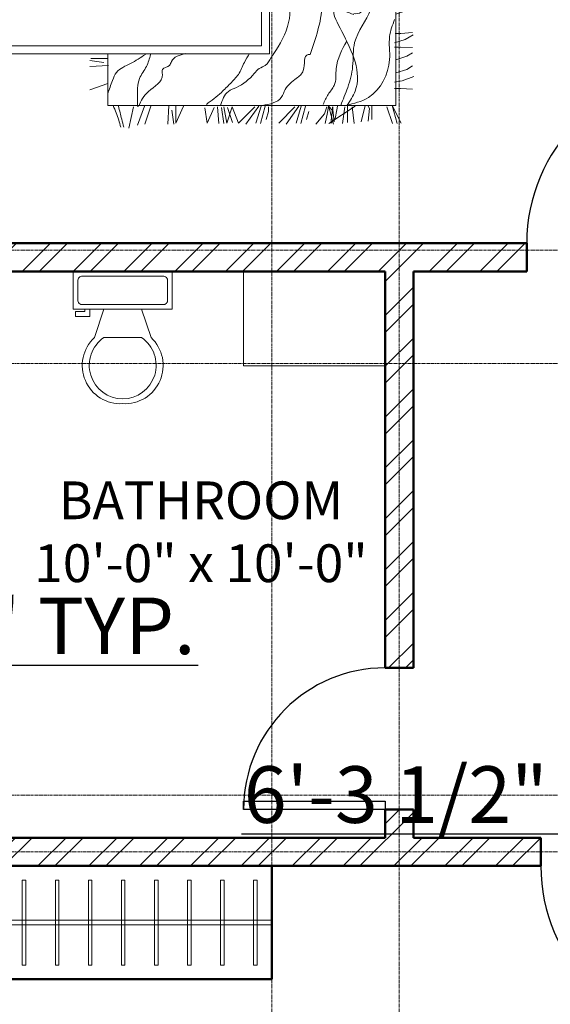
# Model space of a CAD drawing. Units: inches. Extents: x 261 to 2725, y 291 to 1454.
# Tile 21 of 35: x 1295 to 1407, y 644 to 853. Entities that reach past the tile are written whole.
import ezdxf

# ---------------------------------------------------------------- set-up
doc = ezdxf.new("R2010")
doc.units = ezdxf.units.IN
doc.linetypes.add('CENTER', pattern=[2, 1.25, -0.25, 0.25, -0.25])
for name, color, linetype, lineweight in [('A-ANNO-DIMS', 136, 'Continuous', 18), ('A-AREA-IDEN', 18, 'Continuous', 18), ('A-DOOR', 160, 'Continuous', 25), ('A-FLOR-FIXT', 145, 'Continuous', 18), ('A-FURN', 30, 'Continuous', 18), ('A-GRID', 251, 'CENTER', 13), ('A-WALL', 222, 'Continuous', 50), ('A-WALL-PATT', 243, 'Continuous', 13)]:
    doc.layers.add(name, color=color, linetype=linetype, lineweight=lineweight)
doc.styles.get("Standard").update_dxf_attribs({"font": 'arial.ttf'})
doc.dimstyles.new('ISO-25', dxfattribs={"dimtxt": 12, "dimasz": 6, "dimexe": 1.25, "dimexo": 0.625, "dimtad": 1, "dimdec": 0, "dimlunit": 3, "dimtxsty": 'Standard', "dimblk": 'ARCHTICK', "dimcen": 2.5, "dimadec": 0, "dimazin": 0, "dimtfac": 1, "dimtdec": 0, "dimtmove": 0, "dimatfit": 3, "dimfxl": 1, "dimfxlon": 1, "dimarcsym": 0})

# ---------------------------------------------------------------- blocks, each defined once
blk = doc.blocks.new('*U6')
for p, q in [((-36, 0), (-36, 6)), ((0, 0), (0, 6))]:
    blk.add_line(p, q)
blk.add_lwpolyline([(0, 0), (0, -36), (-1.75, -36), (-1.75, 0)], close=True)
blk.add_arc((0, 0), 36, 180, 270)
blk = doc.blocks.new('*U3')
for p, q in [((0, 0), (0, -6)), ((30, 0), (30, -6))]:
    blk.add_line(p, q)
blk.add_lwpolyline([(0, 0), (0, 30), (1.75, 30), (1.75, 0)], close=True)
blk.add_arc((0, 0), 30, 0, 90)
blk = doc.blocks.new('*U7')
for p, q in [((0, 0), (0, -6)), ((-36, 0), (-36, -6))]:
    blk.add_line(p, q)
blk.add_lwpolyline([(0, 0), (0, 36), (-1.75, 36), (-1.75, 0)], close=True)
blk.add_arc((0, 0), 36, 90, 180)
blk = doc.blocks.new('A$C2B723114')
for p, q in [((0, 2.9047), (2.8274, 2.9047)), ((0, 2.8487), (0, 2.9047)), ((2.8274, 2.9047), (2.8274, 2.8487)), ((2.8274, 2.8487), (0, 2.8487)), ((0.1012, 2.4649), (0.1012, 2.849)), ((0.1396, 2.5033), (0.1396, 2.849)), ((0.4243, 2.8697), (0.4243, 2.4855)), ((0.6794, 0.7051), (0.6794, 2.8509)), ((0.7187, 0.7435), (0.7187, 2.8509)), ((2.1776, 2.8509), (2.1776, 0.7454)), ((2.216, 2.8509), (2.216, 0.707)), ((2.4742, 2.8697), (2.4742, 2.4855)), ((2.6798, 2.5052), (2.6798, 2.8509)), ((2.7182, 2.4668), (2.7182, 2.8509)), ((0.6087, 2.6776), (0.295, 2.6776)), ((2.6586, 2.6776), (2.2821, 2.6776)), ((1.3789, 2.4999), (1.3598, 2.5761)), ((2.0593, 2.4999), (2.0402, 2.5761)), ((0.6766, 2.5033), (0.1396, 2.5033)), ((1.3858, 2.4723), (1.3789, 2.4999)), ((2.0662, 2.4723), (2.0593, 2.4999)), ((2.2188, 2.5052), (2.6798, 2.5052)), ((0.6794, 2.4649), (0.1012, 2.4649)), ((0.7191, 2.47), (2.1778, 2.4719)), ((2.2188, 2.4668), (2.7182, 2.4668)), ((2.1771, 2.3036), (0.718, 2.1685)), ((1.0365, 1.6233), (2.1246, 2.2989)), ((2.2287, 1.6076), (2.2523, 1.5035)), ((2.2726, 1.593), (2.3061, 1.5007)), ((2.3067, 1.5881), (2.3373, 1.5007)), ((2.4194, 1.5881), (2.4251, 1.4979)), ((2.4487, 1.5881), (2.4389, 1.5199)), ((0.5047, 1.5819), (0.5353, 1.4945)), ((0.6174, 1.5819), (0.6232, 1.4916)), ((0.6467, 1.5819), (0.6369, 1.5137)), ((0.6571, 1.4945), (0.6571, 1.5765)), ((2.4591, 1.5007), (2.4591, 1.5828)), ((0.4269, 0.0884), (0.4269, 1.4945)), ((0.4269, 1.4945), (0.6794, 1.4945)), ((2.4685, 1.4964), (2.216, 1.5022)), ((2.4685, 1.4964), (2.4685, 0.0903)), ((2.4685, 1.4044), (2.5491, 1.3861)), ((0.3172, 1.3923), (0.4213, 1.3687)), ((0.3318, 1.3485), (0.4241, 1.3149)), ((2.4596, 1.3659), (2.552, 1.3324)), ((0.3367, 1.3143), (0.4241, 1.2838)), ((2.4645, 1.3318), (2.552, 1.3012)), ((2.4645, 1.2928), (2.5548, 1.2871)), ((2.4645, 1.2635), (2.5328, 1.2733)), ((2.4699, 1.2531), (2.552, 1.2163)), ((2.552, 1.2531), (2.4699, 1.2531)), ((2.5435, 1.2276), (2.4699, 1.2163)), ((2.4699, 1.2163), (2.5463, 1.1823)), ((0.3367, 1.2016), (0.427, 1.1959)), ((0.3367, 1.1724), (0.405, 1.1821)), ((0.4241, 1.162), (0.3421, 1.162)), ((0.3421, 1.162), (0.4241, 1.1252)), ((2.5491, 1.1654), (2.467, 1.1597)), ((2.5463, 1.1455), (2.467, 1.1342)), ((2.5491, 1.1342), (2.4699, 1.1201)), ((2.4699, 1.1201), (2.5491, 1.0946)), ((2.5463, 1.1172), (2.4727, 1.0918)), ((2.5491, 1.0946), (2.4699, 1.0635)), ((2.4699, 1.0635), (2.5491, 0.9842)), ((0.4157, 1.0206), (0.3421, 1.0093)), ((2.4642, 1.0267), (2.552, 0.9644)), ((0.3421, 1.0093), (0.4185, 0.9754)), ((2.4699, 0.9785), (2.552, 0.9531)), ((0.4213, 0.9584), (0.3392, 0.9527)), ((0.4185, 0.9386), (0.3392, 0.9272)), ((0.4213, 0.9272), (0.3421, 0.9131)), ((2.4642, 0.9389), (2.4869, 0.9276)), ((2.467, 0.9559), (2.552, 0.9333)), ((2.4869, 0.9276), (2.5265, 0.9163)), ((2.5265, 0.9163), (2.5491, 0.9163)), ((0.3421, 0.9131), (0.4213, 0.8876)), ((0.4213, 0.8876), (0.3421, 0.8565)), ((0.4185, 0.9103), (0.3449, 0.8848)), ((2.4642, 0.8908), (2.5152, 0.8483)), ((0.3364, 0.8197), (0.4241, 0.7574)), ((0.3421, 0.8565), (0.4213, 0.7772)), ((2.467, 0.8455), (2.5208, 0.8342)), ((2.5152, 0.8483), (2.5491, 0.837)), ((2.5208, 0.8342), (2.552, 0.8285)), ((2.552, 0.8285), (2.5293, 0.8087)), ((0.3421, 0.7716), (0.4241, 0.7461)), ((2.5491, 0.7606), (2.467, 0.7719)), ((2.4699, 0.8172), (2.4925, 0.7974)), ((2.5491, 0.8087), (2.4699, 0.8172)), ((2.4925, 0.7974), (2.535, 0.7889)), ((2.535, 0.7889), (2.552, 0.7861)), ((0.3392, 0.7489), (0.4241, 0.7263)), ((2.1776, 0.7454), (0.7187, 0.7435)), ((2.4727, 0.7464), (2.467, 0.7408)), ((2.467, 0.7153), (2.5491, 0.7238)), ((2.552, 0.7464), (2.4727, 0.7464)), ((0.359, 0.7206), (0.3987, 0.7093)), ((0.3987, 0.7093), (0.4213, 0.7093)), ((2.216, 0.707), (0.6794, 0.7051)), ((0.9938, 0.6115), (1.7555, 0.7064)), ((2.5491, 0.6842), (2.4642, 0.6615)), ((2.552, 0.7096), (2.467, 0.6842)), ((0.3421, 0.6601), (0.4213, 0.5808)), ((2.5491, 0.6672), (2.4755, 0.6587)), ((2.4755, 0.6474), (2.5548, 0.6276)), ((0.3364, 0.6233), (0.4241, 0.561)), ((2.4642, 0.6191), (2.4784, 0.6134)), ((2.467, 0.5993), (2.4869, 0.5964)), ((2.4784, 0.6134), (2.5406, 0.6077)), ((2.4869, 0.5964), (2.552, 0.5964)), ((2.5406, 0.6077), (2.552, 0.6134)), ((0.3392, 0.5525), (0.4241, 0.5299)), ((0.3421, 0.5752), (0.4241, 0.5497)), ((2.467, 0.5313), (2.5491, 0.5596)), ((2.467, 0.5087), (2.5548, 0.5342)), ((2.5548, 0.5342), (2.4699, 0.4889)), ((0.359, 0.5242), (0.3987, 0.5129)), ((1.4523, 0.5021), (1.1305, 0.4537)), ((0.3364, 0.4785), (0.3874, 0.436)), ((0.3392, 0.4332), (0.393, 0.4219)), ((0.3874, 0.436), (0.4213, 0.4247)), ((1.1305, 0.4537), (0.9938, 0.448)), ((0.4213, 0.415), (0.3364, 0.3923)), ((0.4241, 0.2868), (0.3392, 0.415)), ((0.3421, 0.4049), (0.3647, 0.3851)), ((0.4213, 0.3964), (0.3421, 0.4049)), ((0.4213, 0.398), (0.3477, 0.3895)), ((0.3647, 0.3851), (0.4072, 0.3766)), ((0.393, 0.4219), (0.4241, 0.4162)), ((0.4241, 0.4162), (0.4015, 0.3964)), ((2.467, 0.4133), (2.552, 0.4019)), ((2.467, 0.2879), (2.552, 0.4076)), ((0.4213, 0.3377), (0.3392, 0.3491)), ((0.4072, 0.3766), (0.4241, 0.3738)), ((0.3392, 0.2925), (0.4213, 0.3009)), ((0.4241, 0.3236), (0.3449, 0.3236)), ((2.4642, 0.3049), (2.5491, 0.2851)), ((2.467, 0.319), (2.5548, 0.3134)), ((0.3477, 0.2571), (0.427, 0.2373)), ((2.4699, 0.2491), (2.501, 0.2491)), ((2.501, 0.2491), (2.5491, 0.2547)), ((0.3506, 0.2231), (0.4128, 0.2175)), ((0.359, 0.2061), (0.4241, 0.2061)), ((0.4128, 0.2175), (0.4241, 0.2231)), ((2.467, 0.2179), (2.5605, 0.1981)), ((2.467, 0.1981), (2.5491, 0.1613)), ((2.467, 0.184), (2.4982, 0.1755)), ((2.4982, 0.1755), (2.5463, 0.1359)), ((0.3392, 0.1042), (0.4213, 0.1325)), ((0.3392, 0.0815), (0.427, 0.107)), ((0.427, 0.107), (0.3421, 0.0617)), ((1.5674, 0.0962), (1.5844, 0.0453)), ((1.8568, 0.0962), (1.8738, 0.0453)), ((1.9342, 0.0962), (1.9512, 0.0453)), ((2.2236, 0.0962), (2.2406, 0.0453)), ((2.4642, 0.0991), (2.5378, 0.0877)), ((2.4699, 0.1302), (2.535, 0.1104)), ((2.535, 0.1104), (2.5491, 0.0991)), ((2.4685, 0.0903), (0.4269, 0.0884)), ((0.5106, 0.0657), (0.5077, 0.0063)), ((0.5106, 0.094), (0.5106, 0.0657)), ((0.5417, 0.094), (0.5474, 0.0572)), ((0.5474, 0.0572), (0.57, 0.0006)), ((0.587, 0.0884), (0.604, 0.0346)), ((0.6512, 0.0884), (0.6682, 0.0346)), ((0.713, 0.0657), (0.7101, 0.0063)), ((0.713, 0.094), (0.713, 0.0657)), ((0.7334, 0.0943), (0.7503, 0.0434)), ((0.7786, 0.0915), (0.7786, 0.0632)), ((0.7786, 0.0632), (0.7843, 0.0066)), ((0.8739, 0.0884), (0.8908, 0.0346)), ((0.956, 0.0943), (0.973, 0.0434)), ((1.0013, 0.0915), (1.0013, 0.0632)), ((1.0013, 0.0632), (1.007, 0.0066)), ((1.072, 0.0884), (1.089, 0.0346)), ((1.1338, 0.0657), (1.131, 0.0063)), ((1.1338, 0.094), (1.1338, 0.0657)), ((1.1542, 0.0943), (1.1712, 0.0434)), ((1.1995, 0.0915), (1.1995, 0.0632)), ((1.1995, 0.0632), (1.2052, 0.0066)), ((1.4088, 0.0657), (1.406, 0.0063)), ((1.4088, 0.094), (1.4088, 0.0657)), ((1.44, 0.094), (1.4456, 0.0572)), ((1.4456, 0.0572), (1.4683, 0.0006)), ((1.4853, 0.0884), (1.5023, 0.0346)), ((1.6127, 0.0934), (1.6127, 0.0651)), ((1.6127, 0.0651), (1.6184, 0.0085)), ((1.6297, 0.0849), (1.624, 0.0028)), ((1.6693, 0.0623), (1.6608, 0.0028)), ((1.6721, 0.0877), (1.6693, 0.0623)), ((1.7344, 0.0651), (1.7316, 0.0057)), ((1.7344, 0.0934), (1.7344, 0.0651)), ((1.7655, 0.0934), (1.7712, 0.0566)), ((1.7712, 0.0566), (1.7938, 0)), ((1.8108, 0.0877), (1.8278, 0.034)), ((1.9795, 0.0934), (1.9795, 0.0651)), ((1.9795, 0.0651), (1.9852, 0.0085)), ((1.9965, 0.0849), (1.9908, 0.0028)), ((2.0361, 0.0623), (2.0276, 0.0028)), ((2.039, 0.0877), (2.0361, 0.0623)), ((2.1012, 0.0651), (2.0984, 0.0057)), ((2.1012, 0.0934), (2.1012, 0.0651)), ((2.1324, 0.0934), (2.138, 0.0566)), ((2.138, 0.0566), (2.1607, 0)), ((2.1777, 0.0877), (2.1946, 0.034)), ((2.2689, 0.0934), (2.2689, 0.0651)), ((2.2689, 0.0651), (2.2746, 0.0085)), ((2.2859, 0.0849), (2.2802, 0.0028)), ((2.3255, 0.0623), (2.317, 0.0028)), ((2.3284, 0.0877), (2.3255, 0.0623)), ((2.3906, 0.0651), (2.3878, 0.0057)), ((2.3906, 0.0934), (2.3906, 0.0651)), ((2.4218, 0.0934), (2.4274, 0.0566)), ((2.4274, 0.0566), (2.4501, 0)), ((2.467, 0.0877), (2.484, 0.034)), ((2.5378, 0.0877), (2.5463, 0.0821)), ((0.604, 0.0346), (0.621, 0.0063)), ((0.6682, 0.0346), (0.6851, 0.0063)), ((0.7503, 0.0434), (0.773, 0.0037)), ((0.8908, 0.0346), (0.9078, 0.0063)), ((0.973, 0.0434), (0.9957, 0.0037)), ((1.089, 0.0346), (1.106, 0.0063)), ((1.1712, 0.0434), (1.1939, 0.0037)), ((1.5023, 0.0346), (1.5192, 0.0082)), ((1.5844, 0.0453), (1.607, 0.0057)), ((1.8278, 0.034), (1.8448, 0.0057)), ((1.8738, 0.0453), (1.8964, 0.0057)), ((1.9512, 0.0453), (1.9739, 0.0057)), ((2.1946, 0.034), (2.2116, 0.0057)), ((2.2406, 0.0453), (2.2632, 0.0057)), ((2.484, 0.034), (2.501, 0.0057))]:
    blk.add_line(p, q)
for centre, radius in [((0.4243, 2.6776), 0.0821), ((2.4742, 2.6776), 0.0821), ((0.4243, 2.6776), 0.0493), ((2.4742, 2.6776), 0.0493)]:
    blk.add_circle(centre, radius)
for centre, radius, start, end in [((0.8078, 2.821), 0.00214, 160.436, 281.8931), ((0.8088, 2.8207), 0.00315, 111.7883, 160.436), ((0.8162, 2.8021), 0.0232, 94.3025, 111.7883), ((0.8091, 2.8151), 0.00394, 21.9904, 101.8931), ((0.8409, 2.7949), 0.0302, 158.579, 188.1335), ((1.0356, 2.8227), 0.2268, 188.1335, 192.1095), ((0.7994, 2.8112), 0.0144, 338.579, 21.9904), ((0.8165, 2.7987), 0.0266, 59.3487, 94.3025), ((0.8554, 2.8643), 0.0497, 239.3487, 264.7408), ((0.9202, 3.5684), 0.7568, 264.7408, 268.0921), ((0.8679, 2.7254), 0.0915, 74.0648, 94.2159), ((0.8679, 2.7254), 0.0915, 53.9136, 74.0648), ((0.9409, 4.189), 1.3777, 268.0921, 270.5757), ((0.8679, 2.7254), 0.0915, 36.1766, 53.9136), ((0.86, 2.6097), 0.2158, 62.7604, 69.1397), ((0.9466, 3.6164), 0.8051, 270.5757, 274.8018), ((0.9263, 2.7386), 0.0708, 51.6114, 62.7604), ((0.7461, 2.511), 0.3611, 46.1885, 51.6114), ((1.0364, 2.548), 0.2671, 87.4614, 94.8018), ((1.042, 2.6745), 0.1405, 79.8101, 87.4614), ((1.1532, 3.2931), 0.488, 259.8101, 263.9133), ((1.204, 3.7695), 0.9671, 263.9133, 270), ((1.204, 3.4318), 0.6294, 270, 277.5469), ((1.2573, 3.0292), 0.2233, 277.5469, 285.744), ((1.3941, 2.5438), 0.281, 98.4372, 105.744), ((1.3747, 2.6748), 0.1486, 90, 98.4372), ((1.3713, 2.8186), 0.0315, 274.4002, 333.4195), ((1.3747, 2.74), 0.0833, 78.7276, 90), ((1.3886, 2.8099), 0.0121, 333.4195, 78.7276), ((1.4882, 2.821), 0.00214, 160.436, 281.8931), ((1.4892, 2.8207), 0.00315, 111.7883, 160.436), ((1.4966, 2.8021), 0.0232, 94.3025, 111.7883), ((1.4895, 2.8151), 0.00394, 21.9904, 101.8931), ((1.5213, 2.7949), 0.0302, 158.579, 188.1335), ((1.716, 2.8227), 0.2268, 188.1335, 192.1095), ((1.4798, 2.8112), 0.0144, 338.579, 21.9904), ((1.4969, 2.7987), 0.0266, 59.3487, 94.3025), ((1.5358, 2.8643), 0.0497, 239.3487, 264.7408), ((1.6006, 3.5684), 0.7568, 264.7408, 268.0921), ((1.5483, 2.7254), 0.0915, 74.0648, 94.2159), ((1.5483, 2.7254), 0.0915, 53.9136, 74.0648), ((1.6213, 4.189), 1.3777, 268.0921, 270.5757), ((1.5483, 2.7254), 0.0915, 36.1766, 53.9136), ((1.5404, 2.6097), 0.2158, 62.7604, 69.1397), ((1.627, 3.6164), 0.8051, 270.5757, 274.8018), ((1.6067, 2.7386), 0.0708, 51.6114, 62.7604), ((1.4265, 2.511), 0.3611, 46.1885, 51.6114), ((1.7168, 2.548), 0.2671, 87.4614, 94.8018), ((1.7224, 2.6745), 0.1405, 79.8101, 87.4614), ((1.8336, 3.2931), 0.488, 259.8101, 263.9133), ((1.8844, 3.7695), 0.9671, 263.9133, 270), ((1.8844, 3.4318), 0.6294, 270, 277.5469), ((1.9377, 3.0292), 0.2233, 277.5469, 285.744), ((2.0745, 2.5438), 0.281, 98.4372, 105.744), ((2.0551, 2.6748), 0.1486, 90, 98.4372), ((2.0517, 2.8186), 0.0315, 274.4002, 333.4195), ((2.0551, 2.74), 0.0833, 78.7276, 90), ((2.069, 2.8099), 0.0121, 333.4195, 78.7276), ((0.635, 2.7368), 0.1829, 7.6809, 12.1095), ((-0.0181, 2.6487), 0.8418, 3.3687, 7.6809), ((0.8679, 2.7254), 0.0915, 18.4397, 36.1766), ((0.8523, 2.6218), 0.2076, 39.0349, 46.1885), ((0.9783, 2.7239), 0.0455, 28.3168, 39.0349), ((0.8558, 2.6579), 0.1846, 23.0028, 28.3168), ((0.923, 2.7382), 0.4535, 0, 6.2324), ((1.3154, 2.7368), 0.1829, 7.6809, 12.1095), ((0.6623, 2.6487), 0.8418, 3.3687, 7.6809), ((1.5483, 2.7254), 0.0915, 18.4397, 36.1766), ((1.5327, 2.6218), 0.2076, 39.0349, 46.1885), ((1.6587, 2.7239), 0.0455, 28.3168, 39.0349), ((1.5362, 2.6579), 0.1846, 23.0028, 28.3168), ((1.6034, 2.7382), 0.4535, 0, 6.2324), ((0.1976, 2.6614), 0.6258, 358.3669, 3.3687), ((0.5722, 2.8434), 0.8132, 347.8016, 350.3156), ((1.1884, 2.7382), 0.1881, 350.3156, 0), ((0.878, 2.6614), 0.6258, 358.3669, 3.3687), ((1.2526, 2.8434), 0.8132, 347.8016, 350.3156), ((1.8688, 2.7382), 0.1881, 350.3156, 0), ((1.9648, 2.5659), 0.6074, 171.9949, 177.3351), ((1.6528, 2.6098), 0.2924, 167.8016, 171.9949), ((2.6452, 2.5659), 0.6074, 171.9949, 177.3351), ((2.3332, 2.6098), 0.2924, 167.8016, 171.9949), ((-11.7321, 3.2823), 12.5718, 356.49514, 356.94504), ((-0.4351, 2.6794), 1.2587, 356.945, 358.3669), ((-11.0517, 3.2823), 12.5718, 356.49514, 356.94504), ((0.2453, 2.6794), 1.2587, 356.945, 358.3669), ((1.4204, 2.5912), 0.0624, 177.3351, 194.0452), ((2.1008, 2.5912), 0.0624, 177.3351, 194.0452), ((0.5206, 2.5319), 0.2961, 350.0016, 356.4951), ((1.4917, 3.1364), 0.681, 244.6889, 246.5156), ((1.4917, 3.1364), 0.681, 246.5156, 248.3423), ((1.4917, 3.1364), 0.681, 248.3423, 250.572), ((1.201, 2.5319), 0.2961, 350.0016, 356.4951), ((2.1721, 3.1364), 0.681, 244.6889, 246.5156), ((2.1721, 3.1364), 0.681, 246.5156, 248.3423), ((2.1721, 3.1364), 0.681, 248.3423, 250.572), ((0.8298, 2.4774), 0.0178, 170.0016, 196.6978), ((0.8139, 2.4726), 0.00122, 196.6978, 277.1204), ((0.8041, 2.5514), 0.0807, 277.1204, 286.2212), ((0.8068, 2.5419), 0.0707, 286.2212, 297.2841), ((0.8584, 2.4419), 0.0418, 102.869, 117.2841), ((0.879, 2.3515), 0.1345, 93.574, 102.869), ((0.9376, 1.4146), 1.0732, 90.2865, 93.574), ((0.9586, -2.7845), 5.2724, 89.0296, 90.2865), ((0.9954, -0.6123), 3.0999, 87.3904, 89.0296), ((1.0854, 1.364), 1.1216, 85.3824, 87.3904), ((1.28, 3.7729), 1.2952, 265.3824, 267.2509), ((1.228, 2.691), 0.2121, 267.2509, 281.5586), ((1.4917, 3.1364), 0.681, 250.572, 252.8018), ((1.2975, 2.3514), 0.1345, 83.5659, 101.5586), ((1.3002, 2.3754), 0.1104, 72.6136, 83.5659), ((1.3965, 2.6828), 0.2118, 252.6136, 260.5159), ((1.4027, 2.7202), 0.2496, 260.5159, 265.9171), ((1.385, 2.4721), 0.000845, 265.9171, 14.0449), ((1.5102, 2.4774), 0.0178, 170.0016, 196.6978), ((1.4943, 2.4726), 0.00122, 196.6978, 277.1204), ((1.4845, 2.5514), 0.0807, 277.1204, 286.2212), ((1.4872, 2.5419), 0.0707, 286.2212, 297.2841), ((1.5388, 2.4419), 0.0418, 102.869, 117.2841), ((1.5594, 2.3515), 0.1345, 93.574, 102.869), ((1.618, 1.4146), 1.0732, 90.2865, 93.574), ((1.639, -2.7845), 5.2724, 89.0296, 90.2865), ((1.6758, -0.6123), 3.0999, 87.3904, 89.0296), ((1.7658, 1.364), 1.1216, 85.3824, 87.3904), ((1.9604, 3.7729), 1.2952, 265.3824, 267.2509), ((1.9084, 2.691), 0.2121, 267.2509, 281.5586), ((2.1721, 3.1364), 0.681, 250.572, 252.8018), ((1.9779, 2.3514), 0.1345, 83.5659, 101.5586), ((1.9806, 2.3754), 0.1104, 72.6136, 83.5659), ((2.0769, 2.6828), 0.2118, 252.6136, 260.5159), ((2.0831, 2.7202), 0.2496, 260.5159, 265.9171), ((2.0654, 2.4721), 0.000845, 265.9171, 14.0449)]:
    blk.add_arc(centre, radius, start, end)
blk.add_ellipse((0.4962, 1.9132), major_axis=(0.4887, -0.4605), ratio=0.503305, start_param=0.491272, end_param=1.591113)
for points, knots in [([(0.6768, 1.3104), (0.6615, 1.3339), (0.6315, 1.3797), (0.604, 1.4501), (0.5417, 1.4748), (0.5064, 1.4871), (0.4848, 1.4945)], [0, 0, 0, 0, 110.980521, 216.571322, 273.316778, 363.252298, 363.252298, 363.252298, 363.252298]), ([(0.427, 1.4678), (0.4036, 1.4582), (0.3693, 1.4441), (0.3335, 1.4344), (0.3221, 1.4313)], [0, 0, 0, 0, 98.452083, 144.639601, 144.639601, 144.639601, 144.639601]), ([(0.4241, 1.4423), (0.4031, 1.437), (0.3691, 1.4284), (0.3351, 1.4199), (0.3221, 1.4167)], [0, 0, 0, 0, 84.638756, 136.955563, 136.955563, 136.955563, 136.955563]), ([(2.5548, 1.4853), (2.5314, 1.4757), (2.5031, 1.4641), (2.4737, 1.4555), (2.4685, 1.454)], [0, 0, 0, 0, 98.452083, 119.481049, 119.481049, 119.481049, 119.481049]), ([(2.552, 1.4598), (2.5309, 1.4545), (2.5031, 1.4475), (2.4753, 1.4406), (2.4685, 1.4389)], [0, 0, 0, 0, 84.638756, 111.94623, 111.94623, 111.94623, 111.94623]), ([(2.2145, 1.4211), (2.233, 1.4246), (2.2636, 1.4303), (2.2761, 1.3837), (2.3429, 1.3967), (2.3949, 1.3342), (2.4474, 1.3031), (2.4698, 1.2898)], [0, 0, 0, 0, 61.886907, 102.717887, 145.699352, 284.082577, 386.765171, 386.765171, 386.765171, 386.765171]), ([(0.6768, 1.286), (0.6567, 1.2911), (0.6145, 1.3017), (0.5543, 1.3533), (0.4816, 1.349), (0.4362, 1.3493), (0.4233, 1.3493)], [0, 0, 0, 0, 80.250278, 168.388677, 295.908361, 346.663112, 346.663112, 346.663112, 346.663112]), ([(0.4233, 1.3445), (0.4367, 1.3385), (0.464, 1.3264), (0.5129, 1.2848), (0.5456, 1.2161), (0.6131, 1.2349), (0.6142, 1.1913), (0.6642, 1.1806), (0.674, 1.144), (0.6817, 1.1154)], [0, 0, 0, 0, 56.745495, 115.23739, 254.956954, 286.678662, 337.828324, 366.201072, 468.500395, 468.500395, 468.500395, 468.500395]), ([(2.2145, 1.319), (2.2295, 1.319), (2.2678, 1.3192), (2.3288, 1.2705), (2.4143, 1.279), (2.4535, 1.2403), (2.4662, 1.2278)], [0, 0, 0, 0, 57.155505, 146.33427, 287.936209, 355.396728, 355.396728, 355.396728, 355.396728]), ([(2.2182, 1.2059), (2.2419, 1.1958), (2.3116, 1.1659), (2.342, 1.0552), (2.4266, 1.0223), (2.4474, 0.9811), (2.462, 0.9684), (2.4698, 0.9616)], [0, 0, 0, 0, 97.73655, 287.59661, 389.176293, 423.403759, 463.679181, 463.679181, 463.679181, 463.679181]), ([(2.3573, 1.127), (2.3656, 1.1759), (2.3758, 1.2352), (2.3371, 1.1853), (2.3602, 1.1713), (2.3768, 1.1612)], [0, 0, 0, 0, 107.853607, 130.728419, 189.220329, 189.220329, 189.220329, 189.220329]), ([(2.2145, 1.1476), (2.2246, 1.1286), (2.2575, 1.0666), (2.3612, 1.0009), (2.431, 0.9336), (2.4662, 0.8996)], [0, 0, 0, 0, 83.02987, 271.460712, 463.033803, 463.033803, 463.033803, 463.033803]), ([(0.6817, 0.8034), (0.6673, 0.8119), (0.6341, 0.8315), (0.5785, 0.8518), (0.5349, 0.8973), (0.4828, 0.9461), (0.4518, 0.9879), (0.4331, 1.013)], [0, 0, 0, 0, 65.318952, 150.437229, 226.833166, 307.58338, 429.454095, 429.454095, 429.454095, 429.454095]), ([(0.4282, 0.9448), (0.4547, 0.9353), (0.496, 0.9206), (0.5223, 0.8436), (0.5628, 0.7946), (0.6113, 0.7575), (0.6214, 0.7173), (0.6539, 0.7022), (0.672, 0.6897), (0.6768, 0.6864)], [0, 0, 0, 0, 102.299436, 159.044876, 303.717955, 348.579152, 391.138254, 454.581655, 477.456496, 477.456496, 477.456496, 477.456496]), ([(2.2145, 0.823), (2.227, 0.8201), (2.261, 0.8121), (2.261, 0.7401), (2.3352, 0.7659), (2.379, 0.6836), (2.4336, 0.6521), (2.4662, 0.6334)], [0, 0, 0, 0, 46.747668, 127.438174, 179.649794, 280.561838, 429.605131, 429.605131, 429.605131, 429.605131]), ([(0.4282, 0.74), (0.4347, 0.7029), (0.444, 0.6496), (0.5194, 0.6274), (0.555, 0.5807), (0.5975, 0.5243), (0.6789, 0.5415), (0.677, 0.5095), (0.6768, 0.5061)], [0, 0, 0, 0, 130.791737, 187.537266, 286.231946, 353.673191, 460.023761, 472.712403, 472.712403, 472.712403, 472.712403]), ([(2.2218, 0.7246), (2.2595, 0.716), (2.3548, 0.6945), (2.4265, 0.6268), (2.4698, 0.586)], [0, 0, 0, 0, 148.665024, 375.555892, 375.555892, 375.555892, 375.555892]), ([(0.6768, 0.6864), (0.7275, 0.655), (0.8251, 0.5944), (0.9391, 0.606), (0.9938, 0.6115)], [0, 0, 0, 0, 225.995823, 434.686543, 434.686543, 434.686543, 434.686543]), ([(2.3719, 0.6737), (2.3738, 0.6431), (2.3772, 0.5878), (2.3146, 0.6382), (2.3401, 0.7015), (2.2971, 0.6649), (2.2923, 0.6965), (2.289, 0.7176)], [0, 0, 0, 0, 83.446591, 150.887818, 201.642461, 230.015204, 286.760644, 286.760644, 286.760644, 286.760644]), ([(2.2145, 0.5167), (2.1764, 0.5522), (2.1051, 0.6184), (1.9357, 0.5803), (1.9385, 0.6342), (1.9388, 0.6395)], [0, 0, 0, 0, 208.073343, 389.01094, 409.01094, 409.01094, 409.01094, 409.01094]), ([(0.6768, 0.5061), (0.7554, 0.4794), (0.8591, 0.4442), (0.9675, 0.4473), (0.9938, 0.448)], [0, 0, 0, 0, 319.374611, 421.61723, 421.61723, 421.61723, 421.61723]), ([(0.4331, 0.4427), (0.4498, 0.4356), (0.4827, 0.4216), (0.5314, 0.3759), (0.632, 0.3884), (0.6996, 0.3513), (0.7423, 0.3278)], [0, 0, 0, 0, 70.931849, 139.556414, 248.154027, 434.709995, 434.709995, 434.709995, 434.709995]), ([(2.4625, 0.1088), (2.4095, 0.1438), (2.2904, 0.2226), (2.0623, 0.1771), (1.9006, 0.2246), (1.7699, 0.2337), (1.6941, 0.2766), (1.5528, 0.2786), (1.4005, 0.2587), (1.2324, 0.3267), (1.059, 0.2939), (0.9218, 0.426), (0.7359, 0.3204), (0.5586, 0.2391), (0.4502, 0.3116), (0.427, 0.3272)], [0, 0, 0, 0, 239.874704, 538.942419, 850.40885, 893.390315, 1047.998294, 1176.505142, 1437.500972, 1637.333004, 1864.324391, 2089.058767, 2248.736533, 2637.953392, 2744.252142, 2744.252142, 2744.252142, 2744.252142]), ([(1.9771, 0.0962), (1.9286, 0.1117), (1.7864, 0.157), (1.5223, 0.1992), (1.2611, 0.141), (1.0527, 0.2023), (0.8859, 0.1885), (0.76, 0.3042), (0.6211, 0.292), (0.5187, 0.3203), (0.4572, 0.3456), (0.4282, 0.3575)], [0, 0, 0, 0, 198.710624, 582.73994, 1031.873213, 1206.082894, 1423.278209, 1655.952104, 1808.744089, 1945.69963, 2068.229211, 2068.229211, 2068.229211, 2068.229211]), ([(0.8718, 0.2941), (0.8821, 0.3221), (0.9041, 0.3814), (0.9523, 0.2773), (0.8733, 0.2454), (0.8757, 0.2798), (0.8766, 0.2941)], [0, 0, 0, 0, 82.720021, 175.094899, 237.579423, 282.440623, 282.440623, 282.440623, 282.440623]), ([(0.8474, 0.0943), (0.82, 0.1047), (0.757, 0.1287), (0.6201, 0.1029), (0.4623, 0.1837), (0.4372, 0.2936), (0.4282, 0.3331)], [0, 0, 0, 0, 112.422038, 258.341957, 533.791494, 688.286079, 688.286079, 688.286079, 688.286079]), ([(1.2715, 0.221), (1.3344, 0.2172), (1.4529, 0.21), (1.2971, 0.2665), (1.2756, 0.2284), (1.2715, 0.221)], [0, 0, 0, 0, 150.888188, 283.977876, 315.699589, 315.699589, 315.699589, 315.699589])]:
    blk.add_open_spline(points, degree=3, knots=knots)
blk = doc.blocks.new('*U27')
for p, q in [((9.5, -6), (9.5, -2)), ((-8, -8.5), (-8, -8)), ((-7, -8), (-7, -9.5)), ((-4, -8), (-6, -14)), ((4, -8), (6, -14)), ((-10, -8.5), (-8, -8.5)), ((-10, -9.5), (-10, -8.5)), ((-7, -9.5), (-10, -9.5)), ((4, -14), (-4, -14))]:
    blk.add_line(p, q)
blk.add_lwpolyline([(10.5, -8), (10.5, 0), (-10.5, 0), (-10.5, -8)], close=True)
for points in [[(-9.5, -2), (-9.5, -6)], [(8.5, -1), (-8.5, -1)], [(-8.5, -7), (8.5, -7)]]:
    blk.add_lwpolyline(points)
for centre, radius, start, end in [((-8.625, -1.875), 0.8839, 81.8699, 188.1301), ((8.625, -1.875), 0.8839, 351.8699, 98.1301), ((-8.625, -6.125), 0.8839, 171.869898, 278.1301), ((8.625, -6.125), 0.8839, 261.8699, 8.1301), ((-0.4772, -19.9188), 8.0953, 133.01722, 273.38), ((0.0374, -19.8731), 7.127, 124.50543, 269.7), ((-0.0373, -19.8731), 7.127, 270.3, 55.4946), ((0.4773, -19.9188), 8.0953, 266.62, 46.9828)]:
    blk.add_arc(centre, radius, start, end)
blk = doc.blocks.new('_ArchTick')
at = {"color": 0, "linetype": 'ByBlock', "const_width": 0.15}
blk.add_lwpolyline([(-0.5, -0.5), (0.5, 0.5)], dxfattribs=at)
blk = doc.blocks.new('*D56')
at = {"layer": 'A-ANNO-DIMS', "color": 0, "lineweight": -2, "ltscale": 0.07, "transparency": 16777216}
for p, q in [((1450.08, 679.22), (1450.08, 681.47)), ((1525.71, 679.22), (1525.71, 681.47)), ((1450.08, 680.22), (1341.66, 680.22)), ((1525.71, 680.22), (1450.08, 680.22))]:
    blk.add_line(p, q, dxfattribs=at)
at = {"layer": 'Defpoints', "color": 0, "ltscale": 0.07, "transparency": 16777216}
for p in [(1450.08, 680.22), (1450.08, 664.47), (1525.71, 664.47)]:
    blk.add_point(p, dxfattribs=at)
at = {"layer": 'A-ANNO-DIMS', "color": 0, "lineweight": -2, "ltscale": 0.07, "transparency": 16777216, "xscale": 6, "yscale": 6, "zscale": 6, "rotation": 180}
blk.add_blockref('_ArchTick', (1450.08, 680.22), dxfattribs=at)
at = {"layer": 'A-ANNO-DIMS', "color": 0, "lineweight": -2, "ltscale": 0.07, "transparency": 16777216, "xscale": 6, "yscale": 6, "zscale": 6}
blk.add_blockref('_ArchTick', (1525.71, 680.22), dxfattribs=at)
at = {"layer": 'A-ANNO-DIMS', "color": 0, "ltscale": 0.07, "transparency": 16777216, "insert": (1392.87, 687.05), "char_height": 12, "attachment_point": 5}
blk.add_mtext('6\'-3 1/2" TYP.', dxfattribs=at)
blk = doc.blocks.new('*D60')
at = {"layer": 'A-ANNO-DIMS', "color": 0, "lineweight": -2, "ltscale": 0.07, "transparency": 16777216}
for p, q in [((1243.08, 717.07), (1243.08, 714.82)), ((1243.08, 716.07), (1252.08, 716.07)), ((1252.08, 717.07), (1252.08, 714.82)), ((1252.08, 716.07), (1332.48, 716.07))]:
    blk.add_line(p, q, dxfattribs=at)
at = {"layer": 'Defpoints', "color": 0, "ltscale": 0.07, "transparency": 16777216}
for p in [(1243.08, 721.47), (1252.08, 721.47), (1252.08, 716.07)]:
    blk.add_point(p, dxfattribs=at)
at = {"layer": 'A-ANNO-DIMS', "color": 0, "lineweight": -2, "ltscale": 0.07, "transparency": 16777216, "xscale": 6, "yscale": 6, "zscale": 6, "rotation": 180}
blk.add_blockref('_ArchTick', (1243.08, 716.07), dxfattribs=at)
at = {"layer": 'A-ANNO-DIMS', "color": 0, "lineweight": -2, "ltscale": 0.07, "transparency": 16777216, "xscale": 6, "yscale": 6, "zscale": 6}
blk.add_blockref('_ArchTick', (1252.08, 716.07), dxfattribs=at)
at = {"layer": 'A-ANNO-DIMS', "color": 0, "ltscale": 0.07, "transparency": 16777216, "insert": (1295.28, 722.82), "char_height": 12, "attachment_point": 5}
blk.add_mtext('0\'-9" TYP.', dxfattribs=at)
blk = doc.blocks.new('*D82')
at = {"layer": 'A-ANNO-DIMS', "color": 0, "lineweight": -2, "ltscale": 0.07, "transparency": 16777216}
for p, q in [((2600.96, 679.47), (2603.21, 679.47)), ((2601.96, 517.47), (2601.96, 679.47)), ((2600.96, 517.47), (2603.21, 517.47))]:
    blk.add_line(p, q, dxfattribs=at)
at = {"layer": 'Defpoints', "color": 0, "ltscale": 0.07, "transparency": 16777216}
for p in [(946.45, 679.47), (2601.96, 679.47), (946.45, 517.47)]:
    blk.add_point(p, dxfattribs=at)
at = {"layer": 'A-ANNO-DIMS', "color": 0, "lineweight": -2, "ltscale": 0.07, "transparency": 16777216, "xscale": 6, "yscale": 6, "zscale": 6}
for p, rotation in [((2601.96, 679.47), 90), ((2601.96, 517.47), 270)]:
    blk.add_blockref('_ArchTick', p, dxfattribs=dict(at, rotation=rotation))
at = {"layer": 'A-ANNO-DIMS', "color": 0, "ltscale": 0.07, "transparency": 16777216, "insert": (2595.2, 598.47), "char_height": 12, "attachment_point": 5, "rotation": 90}
blk.add_mtext('13\'-6"', dxfattribs=at)
blk = doc.blocks.new('*D83')
at = {"layer": 'A-ANNO-DIMS', "color": 0, "lineweight": -2, "ltscale": 0.07, "transparency": 16777216}
for p, q in [((2600.96, 799.47), (2603.21, 799.47)), ((2601.96, 679.47), (2601.96, 799.47)), ((2600.96, 679.47), (2603.21, 679.47))]:
    blk.add_line(p, q, dxfattribs=at)
at = {"layer": 'Defpoints', "color": 0, "ltscale": 0.07, "transparency": 16777216}
for p in [(946.45, 799.47), (2601.96, 799.47), (946.45, 679.47)]:
    blk.add_point(p, dxfattribs=at)
at = {"layer": 'A-ANNO-DIMS', "color": 0, "lineweight": -2, "ltscale": 0.07, "transparency": 16777216, "xscale": 6, "yscale": 6, "zscale": 6}
for p, rotation in [((2601.96, 799.47), 90), ((2601.96, 679.47), 270)]:
    blk.add_blockref('_ArchTick', p, dxfattribs=dict(at, rotation=rotation))
at = {"layer": 'A-ANNO-DIMS', "color": 0, "ltscale": 0.07, "transparency": 16777216, "insert": (2595.21, 739.47), "char_height": 12, "attachment_point": 5, "rotation": 90}
blk.add_mtext('10\'-0"', dxfattribs=at)
blk = doc.blocks.new('*D84')
at = {"layer": 'A-ANNO-DIMS', "color": 0, "lineweight": -2, "ltscale": 0.07, "transparency": 16777216}
for p, q in [((2600.96, 1024.47), (2603.21, 1024.47)), ((2601.96, 799.47), (2601.96, 1024.47)), ((2600.96, 799.47), (2603.21, 799.47))]:
    blk.add_line(p, q, dxfattribs=at)
at = {"layer": 'Defpoints', "color": 0, "ltscale": 0.07, "transparency": 16777216}
for p in [(946.45, 1024.47), (2601.96, 1024.47), (946.45, 799.47)]:
    blk.add_point(p, dxfattribs=at)
at = {"layer": 'A-ANNO-DIMS', "color": 0, "lineweight": -2, "ltscale": 0.07, "transparency": 16777216, "xscale": 6, "yscale": 6, "zscale": 6}
for p, rotation in [((2601.96, 1024.47), 90), ((2601.96, 799.47), 270)]:
    blk.add_blockref('_ArchTick', p, dxfattribs=dict(at, rotation=rotation))
at = {"layer": 'A-ANNO-DIMS', "color": 0, "ltscale": 0.07, "transparency": 16777216, "insert": (2595.21, 911.97), "char_height": 12, "attachment_point": 5, "rotation": 90}
blk.add_mtext('18\'-9"', dxfattribs=at)
blk = doc.blocks.new('*D121')
at = {"layer": 'A-ANNO-DIMS', "color": 0, "lineweight": -2, "ltscale": 0.07, "transparency": 16777216}
for p, q in [((1405.08, 305.22), (1405.08, 302.97)), ((1441.08, 305.22), (1441.08, 302.97)), ((1405.08, 304.22), (1441.08, 304.22))]:
    blk.add_line(p, q, dxfattribs=at)
at = {"layer": 'Defpoints', "color": 0, "ltscale": 0.07, "transparency": 16777216}
for p in [(1405.08, 673.47), (1441.08, 673.47), (1441.08, 304.22)]:
    blk.add_point(p, dxfattribs=at)
at = {"layer": 'A-ANNO-DIMS', "color": 0, "lineweight": -2, "ltscale": 0.07, "transparency": 16777216, "xscale": 6, "yscale": 6, "zscale": 6, "rotation": 180}
blk.add_blockref('_ArchTick', (1405.08, 304.22), dxfattribs=at)
at = {"layer": 'A-ANNO-DIMS', "color": 0, "lineweight": -2, "ltscale": 0.07, "transparency": 16777216, "xscale": 6, "yscale": 6, "zscale": 6}
blk.add_blockref('_ArchTick', (1441.08, 304.22), dxfattribs=at)
at = {"layer": 'A-ANNO-DIMS', "color": 0, "ltscale": 0.07, "transparency": 16777216, "insert": (1423.08, 310.97), "char_height": 12, "attachment_point": 5}
blk.add_mtext('3\'-0"', dxfattribs=at)
blk = doc.blocks.new('*D123')
at = {"layer": 'A-ANNO-DIMS', "color": 0, "lineweight": -2, "ltscale": 0.07, "transparency": 16777216}
for p, q in [((287.06, 1054.85), (284.81, 1054.85)), ((286.06, 439.47), (286.06, 1054.85)), ((287.06, 439.47), (284.81, 439.47))]:
    blk.add_line(p, q, dxfattribs=at)
at = {"layer": 'Defpoints', "color": 0, "ltscale": 0.07, "transparency": 16777216}
for p in [(286.06, 1054.85), (2007.71, 1054.85), (2007.71, 439.47)]:
    blk.add_point(p, dxfattribs=at)
at = {"layer": 'A-ANNO-DIMS', "color": 0, "lineweight": -2, "ltscale": 0.07, "transparency": 16777216, "xscale": 6, "yscale": 6, "zscale": 6}
for p, rotation in [((286.06, 1054.85), 90), ((286.06, 439.47), 270)]:
    blk.add_blockref('_ArchTick', p, dxfattribs=dict(at, rotation=rotation))
at = {"layer": 'A-ANNO-DIMS', "color": 0, "ltscale": 0.07, "transparency": 16777216, "insert": (279.22, 747.16), "char_height": 12, "attachment_point": 5, "rotation": 90}
blk.add_mtext('51\'-3 1/2"', dxfattribs=at)

msp = doc.modelspace()

# ---------------------------------------------------------------- hatches: boundary and pattern name
at = {"layer": 'A-WALL-PATT'}
h = msp.add_hatch(dxfattribs=at)
h.set_pattern_fill('ANSI32', color=256, scale=0.8)
h.paths.add_polyline_path([(478.45, 685.47), (580.45, 685.47), (580.45, 691.47), (577.45, 691.47), (577.45, 694.47), (571.45, 694.47), (571.45, 691.47), (478.45, 691.47), (478.45, 721.47), (469.45, 721.47), (469.45, 508.47), (538.45, 508.47), (538.45, 517.47), (478.45, 517.47)])
h.paths.add_polyline_path([(694.45, 517.47), (676.45, 517.47), (676.45, 646.47), (670.45, 646.47), (670.45, 517.47), (610.45, 517.47), (610.45, 508.47), (694.45, 508.47)])
h.paths.add_polyline_path([(676.45, 784.47), (478.45, 784.47), (478.45, 844.47), (469.45, 844.47), (469.45, 745.47), (478.45, 745.47), (478.45, 775.47), (571.45, 775.47), (571.45, 724.47), (577.45, 724.47), (577.45, 775.47), (670.45, 775.47), (670.45, 691.47), (610.45, 691.47), (610.45, 685.47), (670.45, 685.47), (670.45, 682.47), (676.45, 682.47)])
h.paths.add_polyline_path([(955.45, 880.47), (946.45, 880.47), (946.45, 808.47), (778.45, 808.47), (778.45, 799.47), (946.45, 799.47), (946.45, 517.47), (898.45, 517.47), (898.45, 508.47), (955.45, 508.47)])
h.paths.add_polyline_path([(778.45, 598.47), (772.45, 598.47), (772.45, 517.47), (754.45, 517.47), (754.45, 508.47), (826.45, 508.47), (826.45, 517.47), (778.45, 517.47)])
h.paths.add_polyline_path([(955.45, 1090.47), (946.45, 1090.47), (946.45, 1030.47), (817.45, 1030.47), (817.45, 1024.47), (946.45, 1024.47), (946.45, 952.47), (955.45, 952.47)])
h.paths.add_polyline_path([(955.45, 1231.47), (730.45, 1231.47), (730.45, 1222.47), (772.45, 1222.47), (772.45, 1096.47), (766.45, 1096.47), (766.45, 1090.47), (772.45, 1090.47), (772.45, 1006.47), (712.45, 1006.47), (712.45, 1000.47), (778.45, 1000.47), (778.45, 1024.47), (781.45, 1024.47), (781.45, 1030.47), (778.45, 1030.47), (778.45, 1222.47), (946.45, 1222.47), (946.45, 1162.47), (955.45, 1162.47)])
h.paths.add_polyline_path([(694.45, 1231.47), (619.45, 1231.47), (619.45, 1222.47), (646.45, 1222.47), (646.45, 1039.47), (652.45, 1039.47), (652.45, 1090.47), (736.45, 1090.47), (736.45, 1096.47), (652.45, 1096.47), (652.45, 1222.47), (694.45, 1222.47)])
h.paths.add_polyline_path([(571.45, 1231.47), (469.45, 1231.47), (469.45, 1099.47), (478.45, 1099.47), (478.45, 1144.47), (544.45, 1144.47), (544.45, 1153.47), (538.45, 1153.47), (538.45, 1150.47), (478.45, 1150.47), (478.45, 1222.47), (538.45, 1222.47), (538.45, 1183.47), (544.45, 1183.47), (544.45, 1222.47), (571.45, 1222.47)])
h.paths.add_polyline_path([(538.45, 1006.47), (478.45, 1006.47), (478.45, 1051.47), (469.45, 1051.47), (469.45, 940.47), (478.45, 940.47), (478.45, 1000.47), (538.45, 1000.47)])
h.paths.add_polyline_path([(652.45, 1006.47), (652.45, 1009.47), (646.45, 1009.47), (646.45, 1006.47), (586.45, 1006.47), (586.45, 1000.47), (652.45, 1000.47)])
h.paths.add_polyline_path([(1288.08, 973.47), (1243.08, 973.47), (1243.08, 920.97), (1252.08, 920.97), (1252.08, 964.47), (1288.08, 964.47)], flags=17)
h.paths.add_polyline_path([(1402.08, 805.47), (1252.08, 805.47), (1252.08, 848.97), (1243.08, 848.97), (1243.08, 757.47), (1252.08, 757.47), (1252.08, 799.47), (1294.08, 799.47), (1372.08, 799.47), (1372.08, 779.47), (1372.08, 715.47), (1378.08, 715.47), (1378.08, 799.47), (1402.08, 799.47)])
h.paths.add_polyline_path([(1252.08, 721.47), (1243.08, 721.47), (1243.08, 439.47), (1729.08, 439.47), (1729.08, 709.47), (1720.08, 709.47), (1720.08, 679.47), (1582.08, 679.47), (1582.08, 670.47), (1588.08, 670.47), (1588.08, 673.47), (1720.08, 673.47), (1720.08, 559.47), (1690.08, 559.47), (1690.08, 550.47), (1720.08, 550.47), (1720.08, 448.47), (1252.08, 448.47), (1252.08, 496.47), (1312.08, 496.47), (1312.08, 505.47), (1252.08, 505.47), (1252.08, 673.47), (1405.08, 673.47), (1405.08, 679.47), (1378.08, 679.47), (1378.08, 685.47), (1372.08, 685.47), (1372.08, 679.47), (1252.08, 679.47)])
h.paths.add_polyline_path([(1450.08, 550.47), (1480.08, 550.47), (1480.08, 559.47), (1450.08, 559.47), (1450.08, 679.47), (1441.08, 679.47), (1441.08, 673.47), (1444.08, 673.47), (1444.08, 505.47), (1384.08, 505.47), (1384.08, 496.47), (1450.08, 496.47)], flags=17)
h.paths.add_polyline_path([(1618.08, 559.47), (1588.08, 559.47), (1588.08, 634.47), (1582.08, 634.47), (1582.08, 559.47), (1552.08, 559.47), (1552.08, 550.47), (1618.08, 550.47)], flags=17)
h.paths.add_polyline_path([(1564.08, 964.47), (1630.08, 964.47), (1630.08, 973.47), (1477.08, 973.47), (1477.08, 964.47), (1558.08, 964.47), (1558.08, 926.22), (1558.08, 887.97), (1486.08, 887.97), (1486.08, 881.97), (1558.08, 881.97), (1558.08, 805.47), (1450.08, 805.47), (1450.08, 845.97), (1444.08, 845.97), (1444.08, 805.47), (1438.08, 805.47), (1438.08, 799.47), (1564.08, 799.47)], flags=17)
h.paths.add_polyline_path([(1453.08, 973.47), (1408.08, 973.47), (1408.08, 964.47), (1444.08, 964.47), (1444.08, 881.97), (1450.08, 881.97), (1456.08, 881.97), (1456.08, 887.97), (1450.08, 887.97), (1450.08, 964.47), (1453.08, 964.47)], flags=17)
h.paths.add_polyline_path([(1729.08, 1231.47), (1243.08, 1231.47), (1243.08, 1167.47), (1252.08, 1167.47), (1252.08, 1222.47), (1441.08, 1222.47), (1441.08, 1045.47), (1648.08, 1045.47), (1648.08, 1051.47), (1450.08, 1051.47), (1450.08, 1074.47), (1450.08, 1222.47), (1472.08, 1222.47), (1720.08, 1222.47), (1720.08, 1051.47), (1708.08, 1051.47), (1708.08, 1045.47), (1720.08, 1045.47), (1720.08, 973.47), (1702.08, 973.47), (1702.08, 964.47), (1720.08, 964.47), (1720.08, 769.47), (1729.08, 769.47)])
h.paths.add_polyline_path([(2493.71, 1054.85), (2007.71, 1054.85), (2007.71, 439.47), (2214.67, 439.47), (2214.67, 496.47), (2493.71, 496.47)])
h.paths.add_polyline_path([(2016.71, 1045.85), (2304.71, 1045.85), (2304.71, 841.47), (2310.71, 841.47), (2310.71, 1045.85), (2484.71, 1045.85), (2484.71, 805.47), (2310.71, 805.47), (2310.71, 811.47), (2304.71, 811.47), (2304.71, 799.47), (2484.71, 799.47), (2484.71, 679.47), (2304.71, 679.47), (2304.71, 673.47), (2484.71, 673.47), (2484.71, 505.47), (2208.67, 505.47), (2208.67, 448.47), (2016.71, 448.47), (2016.71, 799.47), (2304.71, 799.47), (2304.71, 805.47), (2016.71, 805.47)], flags=16)

# ---------------------------------------------------------------- linework, layer by layer
at = {"layer": 'A-FLOR-FIXT'}
msp.add_lwpolyline([(1342.08, 779.47), (1372.08, 779.47), (1372.08, 799.47), (1342.08, 799.47)], close=True, dxfattribs=at)
at = {"layer": 'A-FURN'}
for p, q in [((1348.08, 661.97), (1252.08, 661.97)), ((1348.08, 660.97), (1252.08, 660.97))]:
    msp.add_line(p, q, dxfattribs=at)
for points in [[(1295.2, 670.47), (1295.2, 652.47), (1295.95, 652.47), (1295.95, 670.47)], [(1302.2, 670.47), (1302.2, 652.47), (1302.95, 652.47), (1302.95, 670.47)], [(1309.2, 670.47), (1309.2, 652.47), (1309.95, 652.47), (1309.95, 670.47)], [(1316.2, 670.47), (1316.2, 652.47), (1316.95, 652.47), (1316.95, 670.47)], [(1323.2, 670.47), (1323.2, 652.47), (1323.95, 652.47), (1323.95, 670.47)], [(1330.2, 670.47), (1330.2, 652.47), (1330.95, 652.47), (1330.95, 670.47)], [(1337.2, 670.47), (1337.2, 652.47), (1337.95, 652.47), (1337.95, 670.47)], [(1344.2, 670.47), (1344.2, 652.47), (1344.95, 652.47), (1344.95, 670.47)]]:
    msp.add_lwpolyline(points, close=True, dxfattribs=at)
at = {"layer": 'A-GRID', "ltscale": 0.5}
for p, q in [((1348.08, 1330.18), (1348.08, 416.18)), ((1375.08, 1330.18), (1375.08, 416.18)), ((1167.93, 803.97), (1791.93, 803.97)), ((1167.93, 779.97), (1791.93, 779.97)), ((1167.93, 688.47), (1791.93, 688.47)), ((1167.93, 676.47), (1791.93, 676.47))]:
    msp.add_line(p, q, dxfattribs=at)
at = {"layer": 'A-WALL'}
for p, q in [((1252.08, 805.47), (1402.08, 805.47)), ((1402.08, 805.47), (1402.08, 799.47)), ((1252.08, 799.47), (1372.08, 799.47)), ((1372.08, 715.47), (1372.08, 799.47)), ((1378.08, 715.47), (1378.08, 799.47)), ((1378.08, 799.47), (1402.08, 799.47)), ((1378.08, 715.47), (1372.08, 715.47)), ((1372.08, 679.47), (1372.08, 685.47)), ((1378.08, 685.47), (1372.08, 685.47)), ((1378.08, 679.47), (1378.08, 685.47)), ((1252.08, 679.47), (1372.08, 679.47)), ((1378.08, 679.47), (1405.08, 679.47)), ((1405.08, 673.47), (1405.08, 679.47)), ((1252.08, 673.47), (1405.08, 673.47)), ((1348.08, 649.47), (1348.08, 673.47)), ((1252.08, 649.47), (1348.08, 649.47))]:
    msp.add_line(p, q, dxfattribs=at)

# ---------------------------------------------------------------- block references
at = {"layer": 'A-DOOR'}
for name, p in [('*U7', (1438.08, 805.47)), ('*U6', (1441.08, 673.47))]:
    msp.add_blockref(name, p, dxfattribs=at)
at = {"layer": 'A-DOOR', "rotation": 89.99999999999999}
msp.add_blockref('*U3', (1372.08, 685.47), dxfattribs=at)
at = {"layer": 'A-FLOR-FIXT'}
msp.add_blockref('*U27', (1316.47, 799.47), dxfattribs=at)
at = {"layer": 'A-FURN', "xscale": 43.4111919502411, "yscale": 43.4111919502411, "zscale": 43.4111919502411, "rotation": 90}
msp.add_blockref('A$C2B723114', (1378.18, 816.1), dxfattribs=at)

# ---------------------------------------------------------------- texts
at = {"layer": 'A-AREA-IDEN', "insert": (1296.97, 754.98), "char_height": 8, "attachment_point": 1}
msp.add_mtext_dynamic_manual_height_columns('\\pxqc;{\\fTimes New Roman|b0|i0|c0|p18;BATHROOM\\P10\'-0" x 10\'-0"}', width=72.1712, gutter_width=12.5, heights=[0], dxfattribs=at)

# ---------------------------------------------------------------- dimensions: what is measured, and where the dimension line sits
at = {"layer": 'A-ANNO-DIMS', "ltscale": 0.07}
for base, p1, p2, picture, middle in [((286.06, 1054.85), (2007.71, 439.47), (2007.71, 1054.85), '*D123', (279.22, 747.16)), ((2601.96, 1024.47), (946.45, 799.47), (946.45, 1024.47), '*D84', (2595.21, 911.97)), ((2601.96, 799.47), (946.45, 679.47), (946.45, 799.47), '*D83', (2595.21, 739.47)), ((2601.96, 679.47), (946.45, 517.47), (946.45, 679.47), '*D82', (2595.2, 598.47))]:
    dim = msp.add_linear_dim(base=base, p1=p1, p2=p2, angle=90, dimstyle='ISO-25', override={"dimdec": 1, "dimlfac": 1, "dimrnd": 0, "dimzin": 1, "dimdsep": 46, "dimlunit": 4, "dimfrac": 2}, dxfattribs=at)
    dim.commit()
    dim.dimension.update_dxf_attribs({"geometry": picture, "text_midpoint": middle})
dim = msp.add_linear_dim(base=(1252.08, 716.07), p1=(1243.08, 721.47), p2=(1252.08, 721.47), text='<> TYP.', dimstyle='ISO-25', override={"dimdec": 1, "dimrnd": 0, "dimzin": 1, "dimlunit": 4, "dimfrac": 2}, dxfattribs=at)
dim.commit()
dim.dimension.update_dxf_attribs({"geometry": '*D60', "text_midpoint": (1295.28, 722.82)})
dim = msp.add_linear_dim(base=(1450.08, 680.22), p1=(1525.71, 664.47), p2=(1450.08, 664.47), angle=180, text='<> TYP.', dimstyle='ISO-25', override={"dimdec": 1, "dimrnd": 0, "dimzin": 1, "dimlunit": 4, "dimfrac": 2}, dxfattribs=at)
dim.commit()
dim.dimension.update_dxf_attribs({"geometry": '*D56', "text_midpoint": (1392.87, 687.05)})
dim = msp.add_linear_dim(base=(1441.08, 304.22), p1=(1405.08, 673.47), p2=(1441.08, 673.47), dimstyle='ISO-25', override={"dimdec": 1, "dimlfac": 1, "dimrnd": 0, "dimzin": 1, "dimdsep": 46, "dimlunit": 4, "dimfrac": 2}, dxfattribs=at)
dim.commit()
dim.dimension.update_dxf_attribs({"geometry": '*D121', "text_midpoint": (1423.08, 310.97)})

doc.saveas('drawing.dxf')
